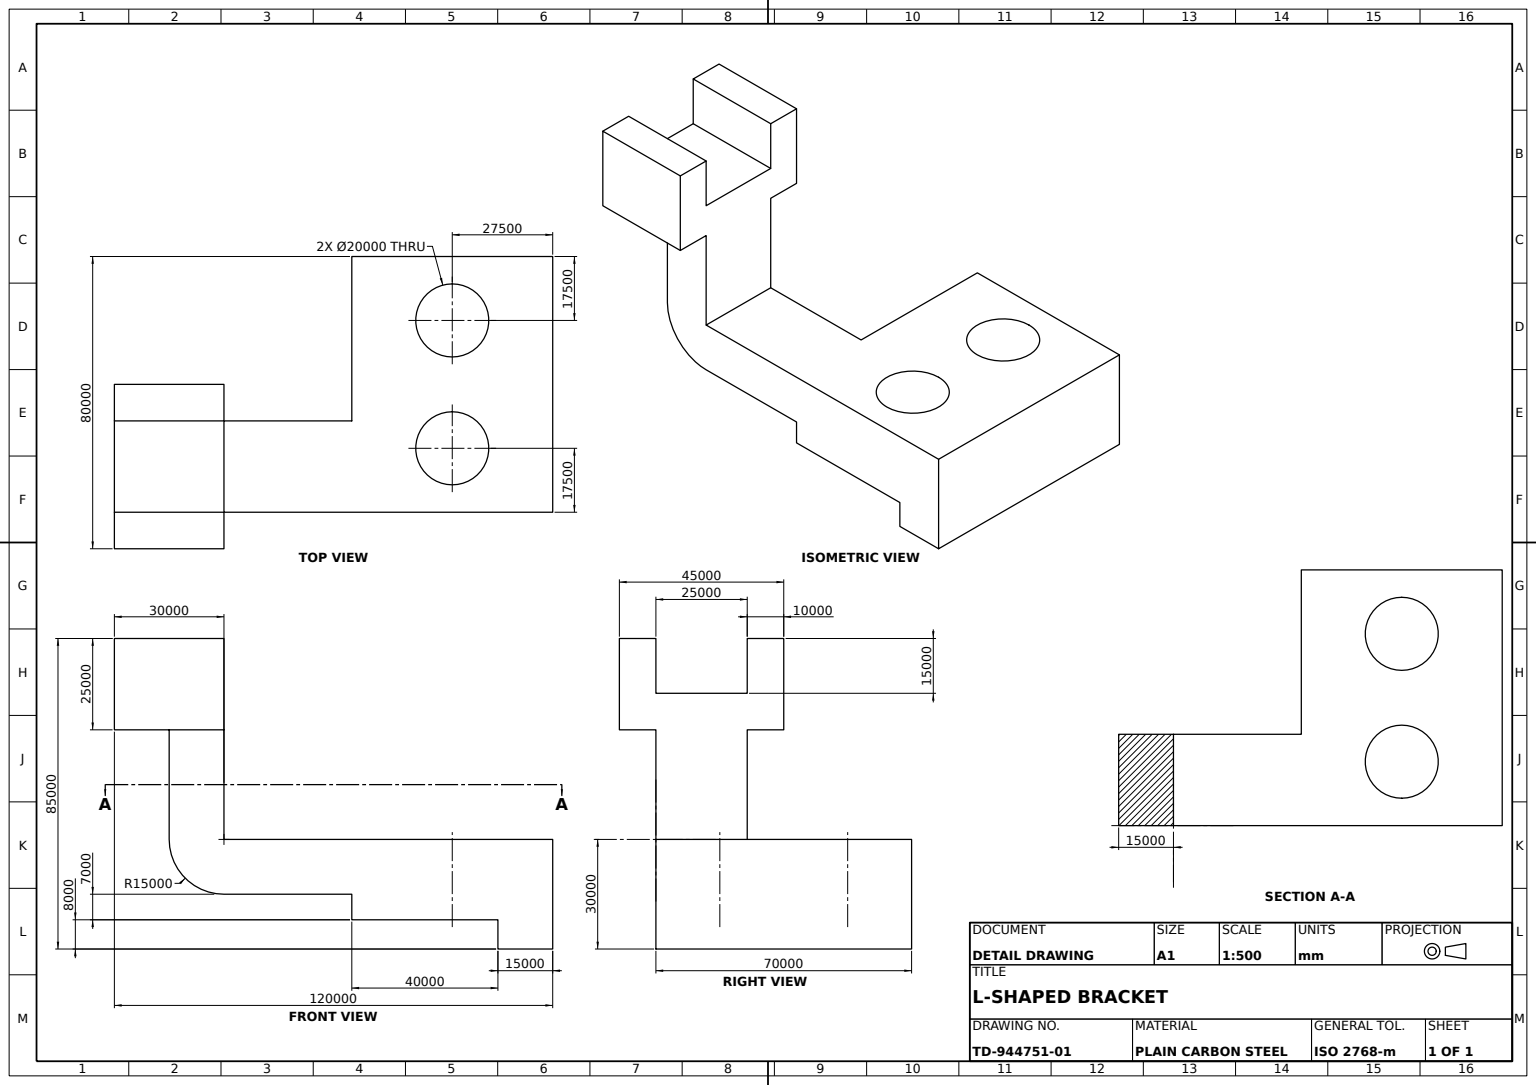
from build123d import *

# Parameters (mm, degrees)
BASE_PLATE_DEPTH           = 35000
UPRIGHT_ARM_SKETCH_W       = 50000
UPRIGHT_ARM_SKETCH_H       = 25000
UPRIGHT_ARM_DEPTH          = 15000
UPRIGHT_EXTENSION_SKETCH_W = 15000
UPRIGHT_EXTENSION_SKETCH_H = 25000
UPRIGHT_EXTENSION_DEPTH    = 30000
BEND_FILLET_R15_R          = 15000
FORK_HEAD_DEPTH            = 30000
MOUNTING_HOLES_SKETCH_R    = 10000
MOUNTING_HOLES_2X_20_DEPTH = 30000


with BuildPart() as part:
    # Base Plate Profile Sketch → Base Plate (new, symmetric)
    with BuildSketch(Plane.XY):
        Polygon((12500, -7000), (-27500, -7000), (-27500, 14474.109792319), (-27500, 15000), (27500, 15000), (27500, -15000), (12500, -15000), align=None)
    extrude(amount=BASE_PLATE_DEPTH, both=True)

    # Upright Arm Sketch → Upright Arm (add)
    with BuildSketch(Plane(origin=(0, 15000, 0), x_dir=(1, 0, 0), z_dir=(0, 1, 0))):
        with Locations((-52500, -22500)):
            Rectangle(UPRIGHT_ARM_SKETCH_W, UPRIGHT_ARM_SKETCH_H)
    extrude(amount=-UPRIGHT_ARM_DEPTH)

    # Upright Extension Sketch → Upright Extension (add)
    with BuildSketch(Plane(origin=(0, 15000, 0), x_dir=(1, 0, 0), z_dir=(0, 1, 0))):
        with Locations((-70000, -22500)):
            Rectangle(UPRIGHT_EXTENSION_SKETCH_W, UPRIGHT_EXTENSION_SKETCH_H)
    extrude(amount=UPRIGHT_EXTENSION_DEPTH)

    # Bend Fillet R15
    bend_fillet_r15_edges = [part.edges().sort_by_distance(p)[0] for p in [
        (-77500, 0, 22500),
    ]]
    fillet(bend_fillet_r15_edges, radius=BEND_FILLET_R15_R)

    # Fork Head Sketch → Fork Head (add)
    with BuildSketch(Plane(origin=(-62500, 0, 0), x_dir=(0, 0, -1), z_dir=(1, 0, 0))):
        Polygon((0, 45000), (-45000, 45000), (-45000, 70000), (-35000, 70000), (-35000, 55000), (-10000, 55000), (-10000, 70000), (0, 70000), align=None)
    extrude(amount=-FORK_HEAD_DEPTH)

    # Mounting Holes Sketch → Mounting Holes 2xØ20 (cut)
    with BuildSketch(Plane(origin=(0, 15000, 0), x_dir=(1, 0, 0), z_dir=(0, 1, 0))):
        with Locations(Location((0, 17500, 0), (0, 0, 270))):
            Circle(MOUNTING_HOLES_SKETCH_R)
        with Locations(Location((0, -17500, 0), (0, 0, 270))):
            Circle(MOUNTING_HOLES_SKETCH_R)
    extrude(amount=-MOUNTING_HOLES_2X_20_DEPTH, mode=Mode.SUBTRACT)


solid = part.part
